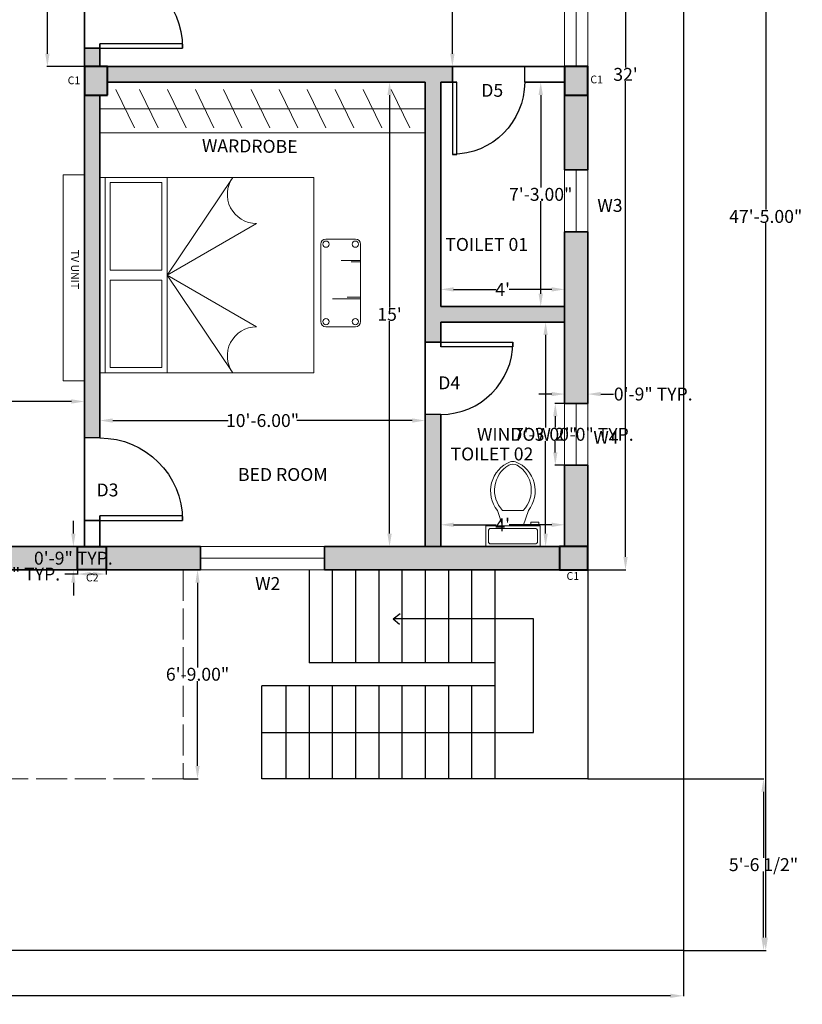
# Model space of a CAD drawing. Units: inches. Extents: x 23868 to 24454, y 31838 to 32477.
# Tile 2 of 4: x 24151 to 24454, y 31851 to 32233. Entities that reach past the tile are written whole.
import ezdxf

# ---------------------------------------------------------------- set-up
doc = ezdxf.new("R2010")
doc.units = ezdxf.units.IN
doc.linetypes.add('ACAD_ISO02W100', pattern=[15, 12, -3])
for name, color, linetype, lineweight in [('A-ANNO-DIMS', 2, 'Continuous', 18), ('A-AREA-IDEN', 7, 'Continuous', 25), ('A-COLS', 7, 'Continuous', 40), ('A-FLOR-CASE', 30, 'Continuous', 18), ('A-FLOR-FIXT', 30, 'Continuous', 18), ('A-FURN', 30, 'Continuous', 18), ('A-GLAZ', 5, 'Continuous', 18), ('A-WALL', 7, 'Continuous', 35), ('C-PROP', 7, 'Continuous', 25), ('door', 1, 'Continuous', 25), ('steps', 104, 'Continuous', 25), ('text', 7, 'Continuous', 18)]:
    doc.layers.add(name, color=color, linetype=linetype, lineweight=lineweight)
for name, color, linetype, lineweight, true_color in [('A-COLS-PATT', 67, 'Continuous', 13, 0x727430), ('A-FLOR-OVHD', 244, 'ACAD_ISO02W100', 18, 0x991b1e), ('A-WALL-PATT', 250, 'Continuous', 13, 0x413a3c)]:
    doc.layers.add(name, color=color, linetype=linetype, lineweight=lineweight, true_color=true_color)
doc.styles.get("Standard").update_dxf_attribs({"font": 'arial.ttf', "height": 5})
doc.styles.add('style1', font='arial.ttf', dxfattribs={"height": 3})
doc.dimstyles.get("Standard").update_dxf_attribs({"dimtxt": 5, "dimasz": 5, "dimexe": 0.18, "dimexo": 0.0625, "dimgap": 0.09, "dimtad": 0, "dimtih": 1, "dimtoh": 1, "dimzin": 0, "dimdsep": 46, "dimlunit": 3, "dimtxsty": 'Standard', "dimcen": 0.09, "dimadec": 0, "dimazin": 0, "dimtfac": 1, "dimtofl": 0, "dimtmove": 0, "dimatfit": 3, "dimfxl": 1, "dimtolj": 1, "dimtzin": 0, "dimarcsym": 0})

# ---------------------------------------------------------------- blocks, each defined once
blk = doc.blocks.new('*U4')
for p, q in [((0, 0), (0, -6)), ((32, 0), (32, -6))]:
    blk.add_line(p, q)
blk.add_lwpolyline([(0, 0), (0, 32), (1.75, 32), (1.75, 0)], close=True)
blk.add_arc((0, 0), 32, 0, 90)
blk = doc.blocks.new('*U5')
for p, q in [((0, 0), (0, -6)), ((28, 0), (28, -6))]:
    blk.add_line(p, q)
blk.add_lwpolyline([(0, 0), (0, 28), (1.75, 28), (1.75, 0)], close=True)
blk.add_arc((0, 0), 28, 0, 90)
blk = doc.blocks.new('NEW BED')
for p, q in [((-75.7, 82.92), (0, 82.92)), ((-75.7, 0), (-75.7, 82.92)), ((-75.7, 80.92), (0, 80.92)), ((0, 82.92), (0, 0)), ((-73.7, 78.92), (-39.85, 78.92)), ((-73.7, 58.92), (-73.7, 78.92)), ((-39.85, 58.92), (-39.85, 78.92)), ((-35.85, 78.92), (-2, 78.92)), ((-35.85, 58.92), (-35.85, 78.92)), ((-2, 78.92), (-2, 58.92)), ((-73.7, 58.92), (-39.85, 58.92)), ((-35.85, 58.92), (-2, 58.92)), ((-75.7, 56.92), (0, 56.92)), ((-37.85, 56.92), (-75.7, 31.45)), ((-37.85, 56.92), (-57.85, 22.27)), ((-37.85, 56.92), (0, 31.45)), ((-37.85, 56.92), (-17.84, 22.27)), ((0, 0), (-75.7, 0))]:
    blk.add_line(p, q)
for centre, start, end in [((-69.14, 22.27), 0, 125.5497), ((-6.56, 22.27), 54.4503, 180)]:
    blk.add_arc(centre, 11.28, start, end)
blk = doc.blocks.new('*U14')
blk.add_line((7.42, 3.61), (-7.42, -3.61))
blk = doc.blocks.new('*U15')
at = {"layer": 'A-FLOR-CASE', "transparency": 16777216}
for p in [(0, 0), (0, -10.83), (0, -21.66), (0, -32.5), (0, -43.33), (0, -54.16), (0, -64.99), (0, -75.82), (0, -86.66), (0, -97.49)]:
    blk.add_blockref('*U14', p, dxfattribs=at)
blk = doc.blocks.new('*D20')
at = {"layer": 'A-ANNO-DIMS', "color": 0, "lineweight": -2, "transparency": 16777216}
for p, q in [((24176.04, 32394.61), (24161.59, 32394.61)), ((24161.77, 32389.61), (24161.77, 32307.25)), ((24161.77, 32219.61), (24161.77, 32301.97)), ((24176.04, 32214.61), (24161.59, 32214.61))]:
    blk.add_line(p, q, dxfattribs=at)
at = {"layer": 'A-ANNO-DIMS', "color": 0, "transparency": 16777216}
for points in [[(24160.94, 32389.61), (24162.6, 32389.61), (24161.77, 32394.61)], [(24160.94, 32219.61), (24162.6, 32219.61), (24161.77, 32214.61)]]:
    blk.add_solid(points, dxfattribs=at)
at = {"layer": 'Defpoints', "color": 0, "transparency": 16777216}
for p in [(24176.1, 32394.61), (24161.77, 32214.61), (24176.1, 32214.61)]:
    blk.add_point(p, dxfattribs=at)
at = {"layer": 'A-ANNO-DIMS', "color": 0, "transparency": 16777216, "insert": (24161.77, 32304.61), "char_height": 5, "attachment_point": 5}
blk.add_mtext("\\A1;15'", dxfattribs=at)
blk = doc.blocks.new('*D22')
at = {"layer": 'A-ANNO-DIMS', "color": 0, "lineweight": -2, "transparency": 16777216}
for p, q in [((24329.04, 32394.61), (24318.46, 32394.61)), ((24318.64, 32389.61), (24318.64, 32307.25)), ((24318.64, 32219.61), (24318.64, 32301.97)), ((24329.04, 32214.61), (24318.46, 32214.61))]:
    blk.add_line(p, q, dxfattribs=at)
at = {"layer": 'A-ANNO-DIMS', "color": 0, "transparency": 16777216}
for points in [[(24317.8, 32389.61), (24319.47, 32389.61), (24318.64, 32394.61)], [(24317.8, 32219.61), (24319.47, 32219.61), (24318.64, 32214.61)]]:
    blk.add_solid(points, dxfattribs=at)
at = {"layer": 'Defpoints', "color": 0, "transparency": 16777216}
for p in [(24329.1, 32394.61), (24318.64, 32214.61), (24329.1, 32214.61)]:
    blk.add_point(p, dxfattribs=at)
at = {"layer": 'A-ANNO-DIMS', "color": 0, "transparency": 16777216, "insert": (24318.64, 32304.61), "char_height": 5, "attachment_point": 5}
blk.add_mtext("\\A1;15'", dxfattribs=at)
blk = doc.blocks.new('*D23')
at = {"layer": 'A-ANNO-DIMS', "color": 0, "lineweight": -2, "transparency": 16777216}
for p, q in [((24297.6, 32208.61), (24294.12, 32208.61)), ((24294.3, 32203.61), (24294.3, 32121.25)), ((24294.3, 32033.61), (24294.3, 32115.97)), ((24297.6, 32028.61), (24294.12, 32028.61))]:
    blk.add_line(p, q, dxfattribs=at)
at = {"layer": 'A-ANNO-DIMS', "color": 0, "transparency": 16777216}
for points in [[(24293.47, 32203.61), (24295.14, 32203.61), (24294.3, 32208.61)], [(24293.47, 32033.61), (24295.14, 32033.61), (24294.3, 32028.61)]]:
    blk.add_solid(points, dxfattribs=at)
at = {"layer": 'Defpoints', "color": 0, "transparency": 16777216}
for p in [(24294.3, 32208.61), (24297.66, 32208.61), (24297.66, 32028.61)]:
    blk.add_point(p, dxfattribs=at)
at = {"layer": 'A-ANNO-DIMS', "color": 0, "transparency": 16777216, "insert": (24294.3, 32118.61), "char_height": 5, "attachment_point": 5}
blk.add_mtext("\\A1;15'", dxfattribs=at)
blk = doc.blocks.new('*D24')
at = {"layer": 'A-ANNO-DIMS', "color": 0, "lineweight": -2, "transparency": 16777216}
for p, q in [((24182.1, 32077.51), (24182.1, 32077.63)), ((24308.1, 32077.51), (24308.1, 32077.63)), ((24187.1, 32077.45), (24231.8, 32077.45)), ((24303.1, 32077.45), (24258.4, 32077.45))]:
    blk.add_line(p, q, dxfattribs=at)
at = {"layer": 'A-ANNO-DIMS', "color": 0, "transparency": 16777216}
for points in [[(24187.1, 32078.28), (24187.1, 32076.61), (24182.1, 32077.45)], [(24303.1, 32078.28), (24303.1, 32076.61), (24308.1, 32077.45)]]:
    blk.add_solid(points, dxfattribs=at)
at = {"layer": 'Defpoints', "color": 0, "transparency": 16777216}
for p in [(24182.1, 32077.45), (24308.1, 32077.45), (24308.1, 32077.45)]:
    blk.add_point(p, dxfattribs=at)
at = {"layer": 'A-ANNO-DIMS', "color": 0, "transparency": 16777216, "insert": (24245.1, 32077.45), "char_height": 5, "attachment_point": 5}
blk.add_mtext('\\A1;10\'-6.00"', dxfattribs=at)
blk = doc.blocks.new('*D25')
at = {"layer": 'A-ANNO-DIMS', "color": 0, "lineweight": -2, "transparency": 16777216}
for p, q in [((24314.1, 32121.67), (24314.1, 32128.46)), ((24319.1, 32128.28), (24335.61, 32128.28)), ((24357.1, 32128.28), (24340.59, 32128.28)), ((24362.1, 32121.67), (24362.1, 32128.46))]:
    blk.add_line(p, q, dxfattribs=at)
at = {"layer": 'A-ANNO-DIMS', "color": 0, "transparency": 16777216}
for points in [[(24319.1, 32129.12), (24319.1, 32127.45), (24314.1, 32128.28)], [(24357.1, 32129.12), (24357.1, 32127.45), (24362.1, 32128.28)]]:
    blk.add_solid(points, dxfattribs=at)
at = {"layer": 'Defpoints', "color": 0, "transparency": 16777216}
for p in [(24362.1, 32128.28), (24314.1, 32121.61), (24362.1, 32121.61)]:
    blk.add_point(p, dxfattribs=at)
at = {"layer": 'A-ANNO-DIMS', "color": 0, "transparency": 16777216, "insert": (24338.1, 32128.28), "char_height": 5, "attachment_point": 5}
blk.add_mtext("\\A1;4'", dxfattribs=at)
blk = doc.blocks.new('*D26')
at = {"layer": 'A-ANNO-DIMS', "color": 0, "lineweight": -2, "transparency": 16777216}
for p, q in [((24362.04, 32208.61), (24352.68, 32208.61)), ((24352.86, 32203.61), (24352.86, 32167.75)), ((24352.86, 32126.61), (24352.86, 32162.46)), ((24362.04, 32121.61), (24352.68, 32121.61))]:
    blk.add_line(p, q, dxfattribs=at)
at = {"layer": 'A-ANNO-DIMS', "color": 0, "transparency": 16777216}
for points in [[(24352.02, 32203.61), (24353.69, 32203.61), (24352.86, 32208.61)], [(24352.02, 32126.61), (24353.69, 32126.61), (24352.86, 32121.61)]]:
    blk.add_solid(points, dxfattribs=at)
at = {"layer": 'Defpoints', "color": 0, "transparency": 16777216}
for p in [(24352.86, 32208.61), (24362.1, 32208.61), (24362.1, 32121.61)]:
    blk.add_point(p, dxfattribs=at)
at = {"layer": 'A-ANNO-DIMS', "color": 0, "transparency": 16777216, "insert": (24352.86, 32165.11), "char_height": 5, "attachment_point": 5}
blk.add_mtext('\\A1;7\'-3.00"', dxfattribs=at)
blk = doc.blocks.new('*D27')
at = {"layer": 'A-ANNO-DIMS', "color": 0, "lineweight": -2, "transparency": 16777216}
for p, q in [((24314.1, 32028.67), (24314.1, 32037.22)), ((24319.1, 32037.04), (24335.61, 32037.04)), ((24357.1, 32037.04), (24340.59, 32037.04)), ((24362.1, 32028.67), (24362.1, 32037.22))]:
    blk.add_line(p, q, dxfattribs=at)
at = {"layer": 'A-ANNO-DIMS', "color": 0, "transparency": 16777216}
for points in [[(24319.1, 32037.88), (24319.1, 32036.21), (24314.1, 32037.04)], [(24357.1, 32037.88), (24357.1, 32036.21), (24362.1, 32037.04)]]:
    blk.add_solid(points, dxfattribs=at)
at = {"layer": 'Defpoints', "color": 0, "transparency": 16777216}
for p in [(24362.1, 32037.04), (24314.1, 32028.61), (24362.1, 32028.61)]:
    blk.add_point(p, dxfattribs=at)
at = {"layer": 'A-ANNO-DIMS', "color": 0, "transparency": 16777216, "insert": (24338.1, 32037.04), "char_height": 5, "attachment_point": 5}
blk.add_mtext("\\A1;4'", dxfattribs=at)
blk = doc.blocks.new('*D28')
at = {"layer": 'A-ANNO-DIMS', "color": 0, "lineweight": -2, "transparency": 16777216}
for p, q in [((24362.04, 32115.61), (24354.57, 32115.61)), ((24354.75, 32110.61), (24354.75, 32074.75)), ((24354.75, 32033.61), (24354.75, 32069.46)), ((24362.04, 32028.61), (24354.57, 32028.61))]:
    blk.add_line(p, q, dxfattribs=at)
at = {"layer": 'A-ANNO-DIMS', "color": 0, "transparency": 16777216}
for points in [[(24353.92, 32110.61), (24355.59, 32110.61), (24354.75, 32115.61)], [(24353.92, 32033.61), (24355.59, 32033.61), (24354.75, 32028.61)]]:
    blk.add_solid(points, dxfattribs=at)
at = {"layer": 'Defpoints', "color": 0, "transparency": 16777216}
for p in [(24362.1, 32115.61), (24354.75, 32028.61), (24362.1, 32028.61)]:
    blk.add_point(p, dxfattribs=at)
at = {"layer": 'A-ANNO-DIMS', "color": 0, "transparency": 16777216, "insert": (24354.75, 32072.11), "char_height": 5, "attachment_point": 5}
blk.add_mtext('\\A1;7\'-3.00"', dxfattribs=at)
blk = doc.blocks.new('*D29')
at = {"layer": 'A-ANNO-DIMS', "color": 0, "lineweight": -2, "transparency": 16777216}
for p, q in [((24214.45, 32019.61), (24220.11, 32019.61)), ((24219.93, 32014.61), (24219.93, 31981.75)), ((24219.93, 31943.61), (24219.93, 31976.47)), ((24214.45, 31938.61), (24220.11, 31938.61))]:
    blk.add_line(p, q, dxfattribs=at)
at = {"layer": 'A-ANNO-DIMS', "color": 0, "transparency": 16777216}
for points in [[(24219.09, 32014.61), (24220.76, 32014.61), (24219.93, 32019.61)], [(24219.09, 31943.61), (24220.76, 31943.61), (24219.93, 31938.61)]]:
    blk.add_solid(points, dxfattribs=at)
at = {"layer": 'Defpoints', "color": 0, "transparency": 16777216}
for p in [(24214.38, 32019.61), (24219.93, 32019.61), (24214.38, 31938.61)]:
    blk.add_point(p, dxfattribs=at)
at = {"layer": 'A-ANNO-DIMS', "color": 0, "transparency": 16777216, "insert": (24219.93, 31979.11), "char_height": 5, "attachment_point": 5}
blk.add_mtext('\\A1;6\'-9.00"', dxfattribs=at)
blk = doc.blocks.new('*D31')
at = {"layer": 'A-ANNO-DIMS', "color": 0, "lineweight": -2, "transparency": 16777216}
for p, q in [((24371.16, 32403.61), (24385.88, 32403.61)), ((24385.7, 32398.61), (24385.7, 32214.25)), ((24385.7, 32024.61), (24385.7, 32208.96)), ((24371.16, 32019.61), (24385.88, 32019.61))]:
    blk.add_line(p, q, dxfattribs=at)
at = {"layer": 'A-ANNO-DIMS', "color": 0, "transparency": 16777216}
for points in [[(24384.86, 32398.61), (24386.53, 32398.61), (24385.7, 32403.61)], [(24384.86, 32024.61), (24386.53, 32024.61), (24385.7, 32019.61)]]:
    blk.add_solid(points, dxfattribs=at)
at = {"layer": 'Defpoints', "color": 0, "transparency": 16777216}
for p in [(24371.1, 32403.61), (24385.7, 32403.61), (24371.1, 32019.61)]:
    blk.add_point(p, dxfattribs=at)
at = {"layer": 'A-ANNO-DIMS', "color": 0, "transparency": 16777216, "insert": (24385.7, 32211.61), "char_height": 5, "attachment_point": 5}
blk.add_mtext("\\A1;32'", dxfattribs=at)
blk = doc.blocks.new('*D33')
at = {"layer": 'A-ANNO-DIMS', "color": 0, "lineweight": -2, "transparency": 16777216}
for p, q in [((23936.1, 32084.78), (23936.1, 32084.66)), ((23941.1, 32084.84), (24051.72, 32084.84)), ((24171.1, 32084.84), (24060.48, 32084.84)), ((24176.1, 32084.9), (24176.1, 32085.02))]:
    blk.add_line(p, q, dxfattribs=at)
at = {"layer": 'A-ANNO-DIMS', "color": 0, "transparency": 16777216}
for points in [[(23941.1, 32085.67), (23941.1, 32084.01), (23936.1, 32084.84)], [(24171.1, 32085.67), (24171.1, 32084.01), (24176.1, 32084.84)]]:
    blk.add_solid(points, dxfattribs=at)
at = {"layer": 'Defpoints', "color": 0, "transparency": 16777216}
for p in [(23936.1, 32084.84), (24176.1, 32084.84), (24176.1, 32084.84)]:
    blk.add_point(p, dxfattribs=at)
at = {"layer": 'A-ANNO-DIMS', "color": 0, "transparency": 16777216, "insert": (24056.1, 32084.84), "char_height": 5, "attachment_point": 5}
blk.add_mtext("\\A1;20'", dxfattribs=at)
blk = doc.blocks.new('*U38')
for p, q in [((9.5, -6), (9.5, -2)), ((-10, -8.5), (-8, -8.5)), ((-10, -9.5), (-10, -8.5)), ((-7, -9.5), (-10, -9.5)), ((-8, -8.5), (-8, -8)), ((-7, -8), (-7, -9.5)), ((-4, -8), (-6, -14)), ((4, -8), (6, -14)), ((4, -14), (-4, -14))]:
    blk.add_line(p, q)
blk.add_lwpolyline([(10.5, -8), (10.5, 0), (-10.5, 0), (-10.5, -8)], close=True)
for points in [[(-9.5, -2), (-9.5, -6)], [(8.5, -1), (-8.5, -1)], [(-8.5, -7), (8.5, -7)]]:
    blk.add_lwpolyline(points)
for centre, radius, start, end in [((-8.62, -1.88), 0.884, 81.8699, 188.1301), ((8.62, -1.88), 0.884, 351.8699, 98.1301), ((-8.62, -6.12), 0.884, 171.8699, 278.1301), ((8.62, -6.12), 0.884, 261.8699, 8.1301), ((3.52, -21.58), 12.17, 141.4691, 247.9714), ((4.2, -21.82), 11.33, 136.3677, 238.9468), ((-3.52, -21.58), 12.17, 292.0284, 38.5307), ((-4.2, -21.82), 11.33, 301.053, 43.6321), ((0, -27.88), 4, 245.7318, 294.2682), ((0, -29), 4, 254.8605, 285.1395)]:
    blk.add_arc(centre, radius, start, end)
blk = doc.blocks.new('*D40')
at = {"layer": 'A-ANNO-DIMS', "color": 0, "lineweight": -2, "transparency": 16777216}
for p, q in [((24408.16, 32441.05), (24440.19, 32441.05)), ((24440.01, 32436.05), (24440.01, 32159.19)), ((24440.01, 31877.05), (24440.01, 32153.91)), ((24408.16, 31872.05), (24440.19, 31872.05))]:
    blk.add_line(p, q, dxfattribs=at)
at = {"layer": 'A-ANNO-DIMS', "color": 0, "transparency": 16777216}
for points in [[(24439.18, 32436.05), (24440.85, 32436.05), (24440.01, 32441.05)], [(24439.18, 31877.05), (24440.85, 31877.05), (24440.01, 31872.05)]]:
    blk.add_solid(points, dxfattribs=at)
at = {"layer": 'Defpoints', "color": 0, "transparency": 16777216}
for p in [(24408.1, 32441.05), (24408.1, 31872.05), (24440.01, 31872.05)]:
    blk.add_point(p, dxfattribs=at)
at = {"layer": 'A-ANNO-DIMS', "color": 0, "transparency": 16777216, "insert": (24440.01, 32156.55), "char_height": 5, "attachment_point": 5}
blk.add_mtext('\\A1;47\'-5.00"', dxfattribs=at)
blk = doc.blocks.new('*D41')
at = {"layer": 'A-ANNO-DIMS', "color": 0, "lineweight": -2, "transparency": 16777216}
for p, q in [((23868.1, 31871.99), (23868.1, 31854.3)), ((24408.1, 31871.99), (24408.1, 31854.3)), ((23873.1, 31854.48), (24133.67, 31854.48)), ((24403.1, 31854.48), (24142.53, 31854.48))]:
    blk.add_line(p, q, dxfattribs=at)
at = {"layer": 'A-ANNO-DIMS', "color": 0, "transparency": 16777216}
for points in [[(23873.1, 31855.32), (23873.1, 31853.65), (23868.1, 31854.48)], [(24403.1, 31855.32), (24403.1, 31853.65), (24408.1, 31854.48)]]:
    blk.add_solid(points, dxfattribs=at)
at = {"layer": 'Defpoints', "color": 0, "transparency": 16777216}
for p in [(23868.1, 31872.05), (24408.1, 31872.05), (23868.1, 31854.48)]:
    blk.add_point(p, dxfattribs=at)
at = {"layer": 'A-ANNO-DIMS', "color": 0, "transparency": 16777216, "insert": (24138.1, 31854.48), "char_height": 5, "attachment_point": 5}
blk.add_mtext("\\A1;45'", dxfattribs=at)
blk = doc.blocks.new('WIN-48IN')
blk.add_line((0, 4.5), (48, 4.5))
blk.add_lwpolyline([(0, 0), (48, 0), (48, 9), (0, 9)], close=True)
blk = doc.blocks.new('WIN-24IN')
blk.add_line((4.5, 0), (4.5, 24))
blk.add_lwpolyline([(0, 24), (9, 24), (9, 0), (0, 0)], close=True)
blk = doc.blocks.new('COL-C1')
blk.add_lwpolyline([(9, 0), (9, 11.01), (0, 11.01), (0, 0)], close=True)
blk = doc.blocks.new('COL-C2')
blk.add_lwpolyline([(11.01, 9), (0, 9), (0, 0), (11.01, 0)], close=True)
blk = doc.blocks.new('*D49')
at = {"layer": 'A-ANNO-DIMS', "color": 0, "lineweight": -2, "transparency": 16777216}
for p, q in [((24173.47, 32017.96), (24168.47, 32017.96)), ((24173.47, 32019.55), (24173.47, 32017.78)), ((24179.48, 32017.96), (24178.47, 32017.96)), ((24184.48, 32019.55), (24184.48, 32017.78))]:
    blk.add_line(p, q, dxfattribs=at)
at = {"layer": 'A-ANNO-DIMS', "color": 0, "transparency": 16777216}
for points in [[(24178.47, 32018.79), (24178.47, 32017.12), (24173.47, 32017.96)], [(24179.48, 32018.79), (24179.48, 32017.12), (24184.48, 32017.96)]]:
    blk.add_solid(points, dxfattribs=at)
at = {"layer": 'Defpoints', "color": 0, "transparency": 16777216}
for p in [(24173.47, 32019.61), (24173.47, 32017.96), (24184.48, 32019.61)]:
    blk.add_point(p, dxfattribs=at)
at = {"layer": 'A-ANNO-DIMS', "color": 0, "transparency": 16777216, "insert": (24129.69, 32017.96), "char_height": 5, "attachment_point": 5}
blk.add_mtext('\\A1;COLUMN C2 0\'-11" TYP.', dxfattribs=at)
blk = doc.blocks.new('*D50')
at = {"layer": 'A-ANNO-DIMS', "color": 0, "lineweight": -2, "transparency": 16777216}
for p, q in [((24171.82, 32033.61), (24171.82, 32038.61)), ((24173.41, 32028.61), (24171.64, 32028.61)), ((24173.41, 32019.61), (24171.64, 32019.61)), ((24171.82, 32014.61), (24171.82, 32009.61))]:
    blk.add_line(p, q, dxfattribs=at)
at = {"layer": 'A-ANNO-DIMS', "color": 0, "transparency": 16777216}
for points in [[(24170.99, 32033.61), (24172.65, 32033.61), (24171.82, 32028.61)], [(24170.99, 32014.61), (24172.65, 32014.61), (24171.82, 32019.61)]]:
    blk.add_solid(points, dxfattribs=at)
at = {"layer": 'Defpoints', "color": 0, "transparency": 16777216}
for p in [(24171.82, 32028.61), (24173.47, 32028.61), (24173.47, 32019.61)]:
    blk.add_point(p, dxfattribs=at)
at = {"layer": 'A-ANNO-DIMS', "color": 0, "transparency": 16777216, "insert": (24171.82, 32024.11), "char_height": 5, "attachment_point": 5}
blk.add_mtext('\\A1;0\'-9" TYP.', dxfattribs=at)
blk = doc.blocks.new('*D53')
at = {"layer": 'A-ANNO-DIMS', "color": 0, "lineweight": -2, "transparency": 16777216}
for p, q in [((24362.04, 32084.11), (24358.32, 32084.11)), ((24358.5, 32079.11), (24358.5, 32074.79)), ((24358.5, 32065.11), (24358.5, 32069.43)), ((24362.04, 32060.11), (24358.32, 32060.11))]:
    blk.add_line(p, q, dxfattribs=at)
at = {"layer": 'A-ANNO-DIMS', "color": 0, "transparency": 16777216}
for points in [[(24357.67, 32079.11), (24359.33, 32079.11), (24358.5, 32084.11)], [(24357.67, 32065.11), (24359.33, 32065.11), (24358.5, 32060.11)]]:
    blk.add_solid(points, dxfattribs=at)
at = {"layer": 'Defpoints', "color": 0, "transparency": 16777216}
for p in [(24358.5, 32084.11), (24362.1, 32084.11), (24362.1, 32060.11)]:
    blk.add_point(p, dxfattribs=at)
at = {"layer": 'A-ANNO-DIMS', "color": 0, "transparency": 16777216, "insert": (24358.5, 32072.11), "char_height": 5, "attachment_point": 5}
blk.add_mtext('\\A1;WINDOW 2\'-0" TYP.', dxfattribs=at)
blk = doc.blocks.new('*D54')
at = {"layer": 'A-ANNO-DIMS', "color": 0, "lineweight": -2, "transparency": 16777216}
for p, q in [((24357.1, 32087.71), (24352.1, 32087.71)), ((24362.1, 32084.17), (24362.1, 32087.89)), ((24371.1, 32084.17), (24371.1, 32087.89)), ((24376.1, 32087.71), (24381.1, 32087.71))]:
    blk.add_line(p, q, dxfattribs=at)
at = {"layer": 'A-ANNO-DIMS', "color": 0, "transparency": 16777216}
for points in [[(24357.1, 32088.54), (24357.1, 32086.87), (24362.1, 32087.71)], [(24376.1, 32088.54), (24376.1, 32086.87), (24371.1, 32087.71)]]:
    blk.add_solid(points, dxfattribs=at)
at = {"layer": 'Defpoints', "color": 0, "transparency": 16777216}
for p in [(24371.1, 32087.71), (24362.1, 32084.11), (24371.1, 32084.11)]:
    blk.add_point(p, dxfattribs=at)
at = {"layer": 'A-ANNO-DIMS', "color": 0, "transparency": 16777216, "insert": (24396.43, 32087.71), "char_height": 5, "attachment_point": 5}
blk.add_mtext('\\A1;0\'-9" TYP.', dxfattribs=at)
blk = doc.blocks.new('*D68')
at = {"layer": 'A-ANNO-DIMS', "color": 0, "lineweight": -2, "transparency": 16777216}
for p, q in [((24371.16, 31938.61), (24439.33, 31938.61)), ((24439.15, 31933.61), (24439.15, 31908)), ((24439.15, 31877.05), (24439.15, 31902.65)), ((24408.16, 31872.05), (24439.33, 31872.05))]:
    blk.add_line(p, q, dxfattribs=at)
at = {"layer": 'A-ANNO-DIMS', "color": 0, "transparency": 16777216}
for points in [[(24438.32, 31933.61), (24439.98, 31933.61), (24439.15, 31938.61)], [(24438.32, 31877.05), (24439.98, 31877.05), (24439.15, 31872.05)]]:
    blk.add_solid(points, dxfattribs=at)
at = {"layer": 'Defpoints', "color": 0, "transparency": 16777216}
for p in [(24371.1, 31938.61), (24408.1, 31872.05), (24439.15, 31872.05)]:
    blk.add_point(p, dxfattribs=at)
at = {"layer": 'A-ANNO-DIMS', "color": 0, "transparency": 16777216, "insert": (24439.15, 31905.33), "char_height": 5, "attachment_point": 5}
blk.add_mtext('\\A1;5\'-6 1/2"', dxfattribs=at)

msp = doc.modelspace()

# ---------------------------------------------------------------- hatches: boundary and pattern name
at = {"layer": 'A-COLS-PATT'}
h = msp.add_hatch(color=256, dxfattribs=at)
h.dxf.hatch_style = 1
h.paths.add_polyline_path([(23938.111, 32028.608), (23927.1, 32028.608), (23927.1, 32019.608), (23938.111, 32019.608)])
h.paths.add_polyline_path([(24049.921, 32028.608), (24038.91, 32028.608), (24038.91, 32019.608), (24049.921, 32019.608)])
h.paths.add_polyline_path([(24184.484, 32028.608), (24173.473, 32028.608), (24173.473, 32019.608), (24184.484, 32019.608)])
h.paths.add_polyline_path([(24371.1, 32028.608), (24360.089, 32028.608), (24360.089, 32019.608), (24371.1, 32019.608)])
h.paths.add_polyline_path([(24371.1, 32214.608), (24362.1, 32214.608), (24362.1, 32203.597), (24371.1, 32203.597)])
h.paths.add_polyline_path([(24185.1, 32214.608), (24176.1, 32214.608), (24176.1, 32203.597), (24185.1, 32203.597)])
h.paths.add_polyline_path([(24062.1, 32216.108), (24051.089, 32216.108), (24051.089, 32207.108), (24062.1, 32207.108)])
h.paths.add_polyline_path([(24371.1, 32403.608), (24360.089, 32403.608), (24360.089, 32394.608), (24371.1, 32394.608)])
h.paths.add_polyline_path([(24187.111, 32403.608), (24176.1, 32403.608), (24176.1, 32394.608), (24187.111, 32394.608)])
h.paths.add_polyline_path([(24065.1, 32403.608), (24056.1, 32403.608), (24056.1, 32392.597), (24065.1, 32392.597)])
h.paths.add_polyline_path([(23936.1, 32403.608), (23927.1, 32403.608), (23927.1, 32392.597), (23936.1, 32392.597)])
h.paths.add_polyline_path([(23936.1, 32214.608), (23927.1, 32214.608), (23927.1, 32203.597), (23936.1, 32203.597)])
at = {"layer": 'A-WALL-PATT'}
h = msp.add_hatch(color=256, dxfattribs=at)
h.dxf.hatch_style = 1
h.paths.add_polyline_path([(24062.1, 32372.393, -0.1373564), (24061.938, 32372.971), (24061.938, 32392.597), (24056.1, 32392.597), (24056.1, 32262.608), (24062.1, 32262.608)])
h.paths.add_polyline_path([(24002.1, 32268.608), (23936.1, 32268.608), (23936.1, 32262.608), (23996.1, 32262.608), (23996.1, 32242.608), (24002.1, 32242.608), (24002.1, 32262.608)])
h.paths.add_polyline_path([(24182.1, 32394.608), (24176.1, 32394.608), (24176.1, 32253.718), (24182.1, 32253.718)])
h.paths.add_polyline_path([(24182.1, 32203.597), (24176.1, 32203.597), (24176.1, 32070.713), (24182.1, 32070.713)])
h.paths.add_polyline_path([(24182.1, 32221.718), (24176.1, 32221.718), (24176.1, 32214.608), (24182.1, 32214.608)])
h.paths.add_polyline_path([(24220.21, 32178.769), (24263.841, 32178.195), (24263.977, 32188.497), (24220.345, 32189.072)], flags=9)
h.paths.add_polyline_path([(24233.842, 32051.215), (24274.374, 32051.215), (24274.374, 32061.519), (24233.842, 32061.519)], flags=9)
h.paths.add_polyline_path([(24179.023, 32045.296), (24190.452, 32045.296), (24190.452, 32055.6), (24179.023, 32055.6)], flags=9)
h = msp.add_hatch(color=256, dxfattribs=at)
h.dxf.hatch_style = 1
h.paths.add_polyline_path([(23969.827, 32028.608), (23938.111, 32028.608), (23938.111, 32019.608), (23969.827, 32019.608)])
h.paths.add_polyline_path([(23936.1, 32034.899), (23931.037, 32034.899), (23927.1, 32034.899), (23927.1, 32028.608), (23936.1, 32028.608)])
h.paths.add_polyline_path([(24038.91, 32028.608), (24017.827, 32028.608), (24017.827, 32019.608), (24038.91, 32019.608)])
h.paths.add_polyline_path([(24064.858, 32028.608), (24049.921, 32028.608), (24049.921, 32019.608), (24064.858, 32019.608)])
h.paths.add_polyline_path([(24173.473, 32028.608), (24136.858, 32028.608), (24136.858, 32025.608), (24136.858, 32019.608), (24173.473, 32019.608)])
h.paths.add_polyline_path([(24221.1, 32028.608), (24184.484, 32028.608), (24184.484, 32019.608), (24221.1, 32019.608)])
h.paths.add_polyline_path([(24360.089, 32028.608), (24269.1, 32028.608), (24269.1, 32019.608), (24360.089, 32019.608)])
h.paths.add_polyline_path([(24314.1, 32079.817), (24308.1, 32079.817), (24308.1, 32028.608), (24314.1, 32028.608)])
h.paths.add_polyline_path([(24371.1, 32060.108), (24362.1, 32060.108), (24362.1, 32028.608), (24371.1, 32028.608)])
h.paths.add_polyline_path([(24371.1, 32150.603), (24362.1, 32150.603), (24362.1, 32084.108), (24371.1, 32084.108)])
h.paths.add_polyline_path([(24362.1, 32121.608), (24314.1, 32121.608), (24314.1, 32208.608), (24318.636, 32208.608), (24318.636, 32214.608), (24185.1, 32214.608), (24185.1, 32208.608), (24308.1, 32208.608), (24308.1, 32107.817), (24314.1, 32107.817), (24314.1, 32115.608), (24362.1, 32115.608)])
h.paths.add_polyline_path([(24371.1, 32203.597), (24362.1, 32203.597), (24362.1, 32174.603), (24371.1, 32174.603)])

# ---------------------------------------------------------------- linework, layer by layer
at = {"layer": 'A-FLOR-CASE'}
for p, q in [((24188.304, 32205.732), (24195.526, 32190.886)), ((24308.1, 32198.309), (24182.1, 32198.309)), ((24182.1, 32188.962), (24308.1, 32188.962)), ((24176.1, 32172.616), (24167.861, 32172.616)), ((24167.861, 32172.616), (24167.861, 32092.886)), ((24167.861, 32092.886), (24176.1, 32092.886))]:
    msp.add_line(p, q, dxfattribs=at)
at = {"layer": 'A-FLOR-OVHD'}
for p, q in [((24214.383, 32019.608), (24214.383, 31938.608)), ((24214.383, 31938.608), (23879.1, 31938.608))]:
    msp.add_line(p, q, dxfattribs=at)
at = {"layer": 'A-FURN'}
for p, q in [((24269.662, 32147.791), (24281.065, 32147.791)), ((24267.662, 32115.79), (24267.662, 32145.791)), ((24283.065, 32145.791), (24283.065, 32115.79)), ((24283.065, 32139.449), (24275.599, 32139.449)), ((24283.065, 32138.95), (24279.441, 32138.95)), ((24283.065, 32124.56), (24272.139, 32124.56)), ((24283.065, 32125.22), (24277.937, 32125.22)), ((24281.065, 32113.79), (24269.662, 32113.79))]:
    msp.add_line(p, q, dxfattribs=at)
for centre in [(24269.662, 32145.791), (24281.065, 32145.791), (24269.662, 32115.79), (24281.065, 32115.79)]:
    msp.add_circle(centre, 1.211, dxfattribs=at)
for centre, start, end in [((24269.662, 32145.791), 90, 180), ((24281.065, 32145.791), 0, 90), ((24269.662, 32115.79), 180, 270), ((24281.065, 32115.79), 270, 0)]:
    msp.add_arc(centre, 2, start, end, dxfattribs=at)
at = {"layer": 'A-WALL'}
for p, q in [((24176.1, 32394.608), (24176.1, 32028.608)), ((24182.1, 32223.468), (24182.1, 32214.608)), ((24176.1, 32221.718), (24182.1, 32221.718)), ((24176.1, 32214.608), (24362.1, 32214.608)), ((24318.636, 32208.608), (24318.636, 32214.608)), ((24362.1, 32214.608), (24371.1, 32214.608)), ((24362.1, 32214.608), (24362.1, 32208.608)), ((24185.1, 32208.608), (24308.1, 32208.608)), ((24308.1, 32208.608), (24308.1, 32028.608)), ((24314.1, 32208.608), (24314.1, 32121.608)), ((24314.1, 32208.608), (24320.386, 32208.608)), ((24346.636, 32208.608), (24362.1, 32208.608)), ((24362.1, 32208.608), (24362.1, 32174.603)), ((24182.1, 32203.597), (24182.1, 32070.713)), ((24362.1, 32174.603), (24371.1, 32174.603)), ((24362.1, 32150.603), (24371.1, 32150.603)), ((24362.1, 32150.603), (24362.1, 32084.108)), ((24314.1, 32121.608), (24362.1, 32121.608)), ((24314.1, 32115.608), (24362.1, 32115.608)), ((24314.1, 32115.608), (24314.1, 32106.067)), ((24308.1, 32107.817), (24314.1, 32107.817)), ((24362.1, 32084.108), (24371.1, 32084.108)), ((24314.1, 32079.817), (24314.1, 32028.608)), ((24362.1, 32060.108), (24371.1, 32060.108)), ((24362.1, 32060.108), (24362.1, 32028.608)), ((24182.1, 32040.463), (24182.1, 32028.608)), ((24176.1, 32038.713), (24182.1, 32038.713)), ((24221.1, 32028.608), (24136.858, 32028.608)), ((24221.1, 32028.608), (24221.1, 32019.608)), ((24362.1, 32028.608), (24269.1, 32028.608)), ((24269.1, 32028.608), (24269.1, 32019.608))]:
    msp.add_line(p, q, dxfattribs=at)
for points in [[(24371.1, 32214.608), (24371.1, 32174.603)], [(24371.1, 32150.603), (24371.1, 32084.108)], [(24371.1, 32060.108), (24371.1, 32019.608), (24269.1, 32019.608)], [(24221.1, 32019.608), (24136.858, 32019.608)]]:
    msp.add_lwpolyline(points, dxfattribs=at)
at = {"layer": 'C-PROP'}
for p, q in [((24408.1, 32441.048), (24408.1, 31872.048)), ((24408.1, 31872.048), (23868.1, 31872.048))]:
    msp.add_line(p, q, dxfattribs=at)
at = {"layer": 'steps'}
for p, q in [((24263.1, 32019.608), (24263.1, 31983.608)), ((24272.1, 32019.608), (24272.1, 31983.608)), ((24281.1, 32019.608), (24281.1, 31983.608)), ((24290.1, 32019.608), (24290.1, 31983.608)), ((24299.1, 32019.608), (24299.1, 31983.608)), ((24308.1, 32019.608), (24308.1, 31983.608)), ((24317.1, 32019.608), (24317.1, 31983.608)), ((24326.1, 32019.608), (24326.1, 31983.608)), ((24335.1, 32019.608), (24335.1, 31983.608)), ((24371.1, 32019.608), (24371.1, 31938.608)), ((24295.739, 32000.593), (24298.415, 32002.615)), ((24350.073, 32000.593), (24295.739, 32000.593)), ((24295.739, 32000.593), (24298.204, 31998.513)), ((24350.073, 31956.608), (24350.073, 32000.593)), ((24335.1, 31983.608), (24335.1, 31974.608)), ((24335.1, 31974.608), (24244.888, 31974.608)), ((24244.888, 31938.608), (24244.888, 31974.608)), ((24254.1, 31974.608), (24254.1, 31938.608)), ((24263.1, 31974.608), (24263.1, 31938.608)), ((24272.1, 31974.608), (24272.1, 31938.608)), ((24281.1, 31974.608), (24281.1, 31938.608)), ((24290.1, 31974.608), (24290.1, 31938.608)), ((24299.1, 31974.608), (24299.1, 31938.608)), ((24308.1, 31974.608), (24308.1, 31938.608)), ((24317.1, 31974.608), (24317.1, 31938.608)), ((24326.1, 31974.608), (24326.1, 31938.608)), ((24335.1, 31974.608), (24335.1, 31938.608)), ((24244.888, 31956.608), (24350.073, 31956.608)), ((24371.1, 31938.608), (24244.888, 31938.608))]:
    msp.add_line(p, q, dxfattribs=at)
msp.add_lwpolyline([(24335.1, 31983.608), (24263.1, 31983.608)], dxfattribs=at)

# ---------------------------------------------------------------- block references
at = {"layer": 'A-COLS'}
for p in [(24176.1, 32203.597), (24362.1, 32203.597)]:
    msp.add_blockref('COL-C1', p, dxfattribs=at)
at = {"layer": 'A-COLS', "extrusion": (0, 0, -1), "zscale": -1}
msp.add_blockref('COL-C2', (-24184.484, 32019.608), dxfattribs=at)
at = {"layer": 'A-COLS', "rotation": 89.999999999988}
msp.add_blockref('COL-C1', (24371.1, 32019.608), dxfattribs=at)
at = {"layer": 'A-FLOR-CASE', "rotation": 90}
msp.add_blockref('*U15', (24201.031, 32198.309), dxfattribs=at)
at = {"layer": 'A-FLOR-FIXT', "rotation": 180}
msp.add_blockref('*U38', (24342.088, 32028.608), dxfattribs=at)
at = {"layer": 'A-FURN', "rotation": 90}
msp.add_blockref('NEW BED', (24265.021, 32171.643), dxfattribs=at)
at = {"layer": 'A-GLAZ', "rotation": 270.0000000000234}
msp.add_blockref('WIN-48IN', (24362.1, 32262.608), dxfattribs=at)
at = {"layer": 'A-GLAZ'}
for p in [(24362.1, 32150.602), (24362.1, 32060.108)]:
    msp.add_blockref('WIN-24IN', p, dxfattribs=at)
at = {"layer": 'A-GLAZ', "extrusion": (0, 0, -1), "zscale": -1, "rotation": 180}
msp.add_blockref('WIN-48IN', (-24221.1, 32028.609), dxfattribs=at)
at = {"layer": 'door', "xscale": -1}
for name, p, rotation in [('*U4', (24182.1, 32221.718), 270), ('*U5', (24318.636, 32208.608), 180), ('*U4', (24182.1, 32038.713), 270)]:
    msp.add_blockref(name, p, dxfattribs=dict(at, rotation=rotation))
at = {"layer": 'door', "rotation": 270}
msp.add_blockref('*U5', (24314.1, 32107.817), dxfattribs=at)

# ---------------------------------------------------------------- texts
at = {"layer": 'A-AREA-IDEN', "char_height": 5, "attachment_point": 1}
for s, width, heights, insert in [('TOILET 01 ', 34.54231, [5.174], (24315.897, 32148.198)), ('TOILET 02', 36.8061, [0], (24317.938, 32066.998)), ('BED ROOM', 47.89207, [0], (24235.604, 32059.034))]:
    msp.add_mtext_dynamic_manual_height_columns(s, width=width, gutter_width=25, heights=heights, dxfattribs=dict(at, insert=insert))
at = {"layer": 'text', "char_height": 3, "attachment_point": 1, "style": 'style1'}
for s, insert in [('C1', (24372.081, 32211.145)), ('C1', (24169.627, 32210.796)), ('C2', (24176.718, 32018.088)), ('C1', (24362.841, 32018.7))]:
    msp.add_mtext_dynamic_manual_height_columns(s, width=6.09517, gutter_width=15, heights=[0], dxfattribs=dict(at, insert=insert))
at = {"layer": 'text', "char_height": 5, "attachment_point": 1}
for s, insert in [('D5', (24329.837, 32207.929)), ('W3', (24374.779, 32163.313)), ('D4', (24313.174, 32094.561)), ('W4', (24373.239, 32073.444)), ('D3', (24180.812, 32053.047)), ('W2', (24242.232, 32016.774))]:
    msp.add_mtext_dynamic_manual_height_columns(s, width=9.30203, gutter_width=12.5, heights=[0], dxfattribs=dict(at, insert=insert))
at = {"layer": 'text', "insert": (24221.648, 32186.57), "char_height": 5, "attachment_point": 1, "rotation": 359.24585}
msp.add_mtext_dynamic_manual_height_columns('WARDROBE', width=25.67088, gutter_width=25, heights=[0], dxfattribs=at)
at = {"layer": 'text', "insert": (24173.959, 32143.647), "char_height": 3, "attachment_point": 1, "rotation": 270, "style": 'style1'}
msp.add_mtext_dynamic_manual_height_columns('TV UNIT', width=35.25869, gutter_width=15, heights=[0], dxfattribs=at)

# ---------------------------------------------------------------- dimensions: what is measured, and where the dimension line sits
at = {"layer": 'A-ANNO-DIMS'}
for base, p1, p2, override, picture, middle in [((24440.012, 31872.048), (24408.1, 32441.048), (24408.1, 31872.048), {"dimclrd": 0, "dimclre": 0, "dimclrt": 0}, '*D40', (24440.012, 32156.548)), ((24385.697, 32403.608), (24371.1, 32019.608), (24371.1, 32403.608), {"dimclrd": 0, "dimclre": 0, "dimclrt": 0}, '*D31', (24385.697, 32211.608)), ((24161.769, 32214.608), (24176.1, 32394.608), (24176.1, 32214.608), {"dimclrd": 0, "dimclre": 0, "dimclrt": 0}, '*D20', (24161.769, 32304.608)), ((24318.636, 32214.608), (24329.1, 32394.608), (24329.1, 32214.608), {"dimclrd": 0, "dimclre": 0, "dimclrt": 0}, '*D22', (24318.636, 32304.608)), ((24294.303, 32208.608), (24297.662, 32028.608), (24297.662, 32208.608), {"dimclrd": 0, "dimclre": 0, "dimclrt": 0}, '*D23', (24294.303, 32118.608)), ((24352.857, 32208.608), (24362.1, 32121.608), (24362.1, 32208.608), {"dimclrd": 0, "dimclre": 0, "dimclrt": 0}, '*D26', (24352.857, 32165.108)), ((24354.753, 32028.608), (24362.1, 32115.608), (24362.1, 32028.608), {"dimclrd": 0, "dimclre": 0, "dimclrt": 0}, '*D28', (24354.753, 32072.108)), ((24219.926, 32019.608), (24214.383, 31938.608), (24214.383, 32019.608), {"dimclrd": 0, "dimclre": 0, "dimclrt": 0}, '*D29', (24219.926, 31979.108)), ((24439.15, 31872.048), (24371.1, 31938.608), (24408.1, 31872.048), {"dimdec": 1, "dimlfac": 1, "dimrnd": 0, "dimzin": 1, "dimdsep": 46, "dimlunit": 4, "dimfrac": 2}, '*D68', (24439.15, 31905.328))]:
    dim = msp.add_linear_dim(base=base, p1=p1, p2=p2, angle=90, dimstyle='Standard', override=override, dxfattribs=at)
    dim.commit()
    dim.dimension.update_dxf_attribs({"geometry": picture, "text_midpoint": middle})
for base, p1, p2, picture, middle in [((24362.1, 32128.284), (24314.1, 32121.608), (24362.1, 32121.608), '*D25', (24338.1, 32128.284)), ((24176.1, 32084.84), (23936.1, 32084.84), (24176.1, 32084.84), '*D33', (24056.1, 32084.84)), ((24308.1, 32077.447), (24182.1, 32077.447), (24308.1, 32077.447), '*D24', (24245.1, 32077.447)), ((24362.1, 32037.045), (24314.1, 32028.608), (24362.1, 32028.608), '*D27', (24338.1, 32037.045)), ((23868.1, 31854.482), (24408.1, 31872.048), (23868.1, 31872.048), '*D41', (24138.1, 31854.482))]:
    dim = msp.add_linear_dim(base=base, p1=p1, p2=p2, dimstyle='Standard', override={"dimclrd": 0, "dimclre": 0, "dimclrt": 0}, dxfattribs=at)
    dim.commit()
    dim.dimension.update_dxf_attribs({"geometry": picture, "text_midpoint": middle})
dim = msp.add_linear_dim(base=(24371.1, 32087.708), p1=(24362.1, 32084.108), p2=(24371.1, 32084.108), text='<> TYP.', dimstyle='Standard', override={"dimdec": 1, "dimlfac": 1, "dimrnd": 0, "dimzin": 1, "dimdsep": 46, "dimlunit": 4, "dimfrac": 2}, dxfattribs=at)
dim.commit()
dim.dimension.update_dxf_attribs({"geometry": '*D54', "text_midpoint": (24396.429, 32087.708)})
for base, p1, p2, angle, text, picture, middle in [((24358.5, 32084.108), (24362.1, 32060.108), (24362.1, 32084.108), 90, 'WINDOW <> TYP.', '*D53', (24358.5, 32072.108)), ((24171.822, 32028.608), (24173.473, 32019.608), (24173.473, 32028.608), 90, '<> TYP.', '*D50', (24171.822, 32024.108)), ((24173.473, 32017.957), (24184.484, 32019.608), (24173.473, 32019.608), 180, 'COLUMN C2 <> TYP.', '*D49', (24129.691, 32017.957))]:
    dim = msp.add_linear_dim(base=base, p1=p1, p2=p2, angle=angle, text=text, dimstyle='Standard', override={"dimdec": 1, "dimlfac": 1, "dimrnd": 0, "dimzin": 1, "dimdsep": 46, "dimlunit": 4, "dimfrac": 2}, dxfattribs=at)
    dim.commit()
    dim.dimension.update_dxf_attribs({"geometry": picture, "text_midpoint": middle})

doc.saveas('drawing.dxf')
